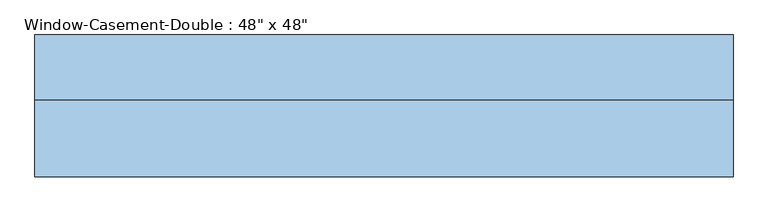
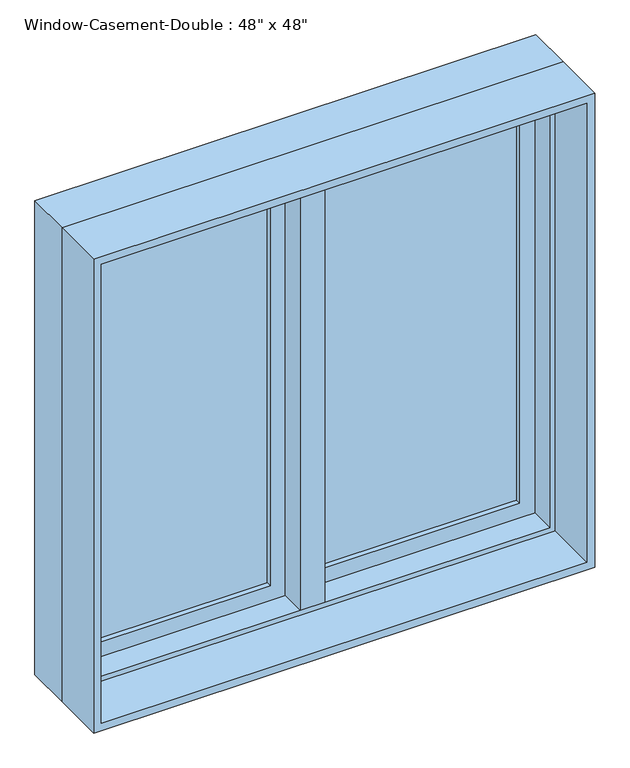
"""IFC4 building model written with IfcOpenShell, lengths in millimetres: window geometry."""

from ifc_helpers import new_model, si_unit, frame, origin, place, context, project, spatial, polyline, outline, extrude, faceted_brep, source, transform, mapped, element, save


def window_af3140d2(model_context):
    return source(origin(), model_context, "Body", "SolidModel", [
        faceted_brep([(9.525, 133.35, 2120.9), (-9.525, 133.35, 2120.9), (-9.525, 82.55, 2120.9), (9.525, 82.55, 2120.9), (9.525, 133.35, 927.1), (9.525, 82.55, 927.1), (-9.525, 82.55, 927.1), (-9.525, 133.35, 927.1), (-9.525, 82.55, 946.15), (-9.525, 82.55, 2101.85), (-30.1625, 82.55, 946.15), (-30.1625, 82.55, 2101.85), (-30.1625, 19.05, 946.15), (-30.1625, 19.05, 2101.85), (30.1625, 19.05, 946.15), (30.1625, 19.05, 2101.85), (30.1625, 82.55, 946.15), (30.1625, 82.55, 2101.85), (9.525, 82.55, 946.15), (9.525, 82.55, 2101.85)], [[[0, 1, 2, 3]], [[4, 5, 6, 7]], [[1, 0, 4, 7]], [[2, 1, 7, 6, 8, 9]], [[9, 8, 10, 11]], [[11, 10, 12, 13]], [[13, 12, 14, 15]], [[15, 14, 16, 17]], [[17, 16, 18, 19]], [[0, 3, 19, 18, 5, 4]], [[18, 8, 6, 5]], [[9, 19, 3, 2]], [[8, 18, 16, 14, 12, 10]], [[19, 9, 11, 13, 15, 17]]]),
        extrude(outline(polyline([(-66.675, 114.3), (-66.675, 107.95), (-539.75, 107.95), (-539.75, 114.3), (-66.675, 114.3)])), frame((0.0, 0.0, 984.25), z_axis=(0.0, 0.0, 1.0), x_axis=(1.0, 0.0, 0.0)), (0.0, 0.0, 1.0), 1079.5),
        extrude(outline(polyline([(-539.75, 95.25), (-539.75, 101.6), (-66.675, 101.6), (-66.675, 95.25), (-539.75, 95.25)])), frame((0.0, 0.0, 984.25), z_axis=(0.0, 0.0, 1.0), x_axis=(1.0, 0.0, 0.0)), (0.0, 0.0, 1.0), 1079.5),
        extrude(outline(polyline([(539.75, 114.3), (539.75, 107.95), (66.675, 107.95), (66.675, 114.3), (539.75, 114.3)])), frame((0.0, 0.0, 984.25), z_axis=(0.0, 0.0, 1.0), x_axis=(1.0, 0.0, 0.0)), (0.0, 0.0, 1.0), 1079.5),
        extrude(outline(polyline([(66.675, 95.25), (66.675, 101.6), (539.75, 101.6), (539.75, 95.25), (66.675, 95.25)])), frame((0.0, 0.0, 984.25), z_axis=(0.0, 0.0, 1.0), x_axis=(1.0, 0.0, 0.0)), (0.0, 0.0, 1.0), 1079.5),
        extrude(outline(polyline([(2120.9, -596.9), (927.1, -596.9), (927.1, -9.525), (2120.9, -9.525), (2120.9, -596.9)]), holes=[polyline([(2063.75, -66.675), (984.25, -66.675), (984.25, -539.75), (2063.75, -539.75), (2063.75, -66.675)])]), frame((0.0, 82.55, 0.0), z_axis=(0.0, 1.0, 0.0), x_axis=(0.0, 0.0, 1.0)), (0.0, 0.0, 1.0), 44.45),
        extrude(outline(polyline([(927.1, 596.9), (2120.9, 596.9), (2120.9, 9.525), (927.1, 9.525), (927.1, 596.9)]), holes=[polyline([(984.25, 66.675), (2063.75, 66.675), (2063.75, 539.75), (984.25, 539.75), (984.25, 66.675)])]), frame((0.0, 82.55, 0.0), z_axis=(0.0, 1.0, 0.0), x_axis=(0.0, 0.0, 1.0)), (0.0, 0.0, 1.0), 44.45),
        extrude(outline(polyline([(2133.6, -609.6), (914.4, -609.6), (914.4, 609.6), (2133.6, 609.6), (2133.6, -609.6)]), holes=[polyline([(2114.55, 590.55), (933.45, 590.55), (933.45, -590.55), (2114.55, -590.55), (2114.55, 590.55)])]), frame((0.0, -114.3, 0.0), z_axis=(0.0, 1.0, 0.0), x_axis=(0.0, 0.0, 1.0)), (0.0, 0.0, 1.0), 133.35),
        faceted_brep([(577.85, 82.55, 2101.85), (577.85, 19.05, 2101.85), (-577.85, 19.05, 2101.85), (-577.85, 82.55, 2101.85), (596.9, 133.35, 2120.9), (596.9, 82.55, 2120.9), (-596.9, 82.55, 2120.9), (-596.9, 133.35, 2120.9), (609.6, 19.05, 2133.6), (609.6, 133.35, 2133.6), (-609.6, 133.35, 2133.6), (-609.6, 19.05, 2133.6), (-577.85, 19.05, 946.15), (-577.85, 82.55, 946.15), (-596.9, 82.55, 927.1), (-596.9, 133.35, 927.1), (-609.6, 133.35, 914.4), (-609.6, 19.05, 914.4), (577.85, 19.05, 946.15), (577.85, 82.55, 946.15), (596.9, 82.55, 927.1), (596.9, 133.35, 927.1), (609.6, 133.35, 914.4), (609.6, 19.05, 914.4)], [[[0, 1, 2, 3]], [[4, 5, 6, 7]], [[8, 9, 10, 11]], [[3, 2, 12, 13]], [[7, 6, 14, 15]], [[11, 10, 16, 17]], [[13, 12, 18, 19]], [[15, 14, 20, 21]], [[17, 16, 22, 23]], [[11, 17, 23, 8], [1, 18, 12, 2]], [[19, 18, 1, 0]], [[5, 20, 14, 6], [3, 13, 19, 0]], [[21, 20, 5, 4]], [[23, 22, 9, 8]], [[9, 22, 16, 10], [7, 15, 21, 4]]]),
    ])


if __name__ == "__main__":
    model = new_model("IFC4")
    model_context = context("Model", 3, world=origin())
    ifc_project = project(units=[si_unit("LENGTHUNIT", "METRE", prefix="MILLI")], contexts=[model_context])
    site = spatial("IfcSite", under=ifc_project)
    building = spatial("IfcBuilding", under=site)
    placement = place(None, origin())
    window_shape = window_af3140d2(model_context)
    element("IfcWindow", 1, ObjectType="Window-Casement-Double : 48\" x 48\"", at=placement, inside=building, context=model_context, shape_type="MappedRepresentation", body=[
        mapped(window_shape, transform((0.0, 0.0, 0.0), x_axis=(1.0, 0.0, 0.0), y_axis=(0.0, 1.0, 0.0), z_axis=(0.0, 0.0, 1.0))),
    ])
    save(model, "model.ifc")

# Revit data of these elements
# Type "Window-Casement-Double : 48\" x 48\""
#   Type Mark = "16"
#   Fire Rating = "0.5h"
#   Assembly Code = "B2020100"
#   Analytic Construction = "Double glazing - domestic"
#   Frame Extension [instance default] = 0' - 0 1/4"
#   Window Inset [instance default] = 0' - 0"
#   Wall Thickness [instance default] = 0' - 6"
#   Interior Wall Closure [instance default] = 0' - 2 1/4"
#   Half Width = 2' - 0"
#   Visual Light Transmittance = 0.81
#   Thermal Resistance (R) = 1.8146 (h·ft²·°F)/BTU
#   Solar Heat Gain Coefficient = 0.76
#   Rough Width = 4' - 0 1/2"
#   Rough Height = 4' - 0 1/2"
#   Height = 4' - 0"
#   Heat Transfer Coefficient (U) = 0.5511 BTU/(h·ft²·°F)
#   Exterior Wall Closure [instance default] = 0' - 1 1/4"
#   Extension Jamb [instance default] = 0' - 2 1/4"
#   Default Sill Height = 3' - 0"
#   Width = 4' - 0"
#   Define Thermal Properties by = 0
#   Muntin Visibility = yes
#   Interior Trim Visibility [instance default] = yes
#   Exterior Trim Visibility [instance default] = yes
#   Extension Jamb Visibility [instance default] = yes
#   Interior Trim Material = Wood - Stained
#   Muntin Pattern = Muntin Pattern_2x2 : Muntin Pattern_2x2
#   Interior Trim = Trim-Window-Interior-Flat : Picture Frame
#   Interior Frame Material = Wood - Stained
#   Glass Panel Material = Glass
#   Exterior Trim Material = Clad - White
#   Exterior Trim = Trim-Window-Exterior-Flat : with Sill
#   Exterior Frame Material = Clad - White
#   Wall Closure = (empty or 0)
# Element 1 (IfcWindow, "Window-Casement-Double : 48\" x 48\"")
#   Wall Thickness = 0' - 9"
#   Extension Jamb = 0' - 5 1/4"
#   Materials on its faces: "Wood - Stained", "Glass", "Clad - White"
# Materials
#   "Wood - Stained": class "Wood", colour RGB 224 178 126, transparency 0, Cost = 0
#   "Glass": class "Glass", colour RGB 0 128 192, transparency 0.75, Description = "Soda Lime Glass", Cost = 0
#   "Clad - White": class "Wood", colour RGB 242 242 238, transparency 0, Cost = 0
